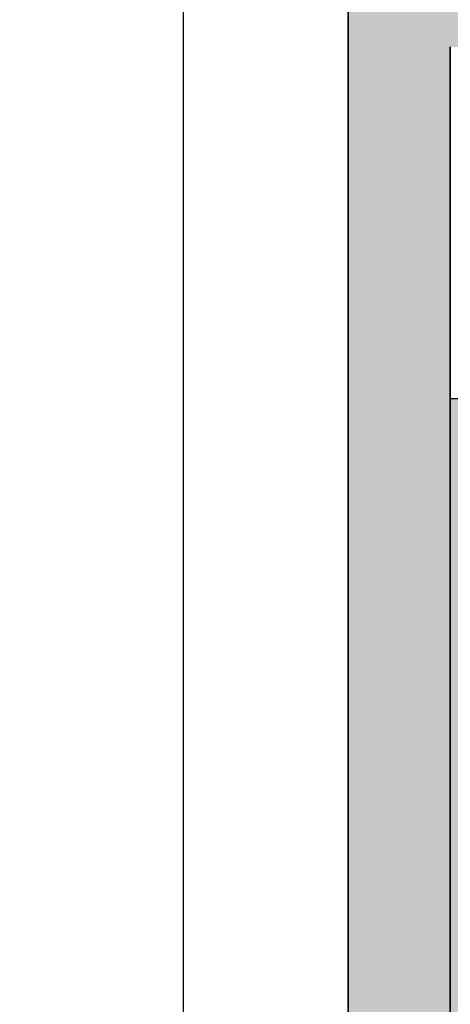
# Model space of a CAD drawing. Units: inches. Extents: x 3592 to 4861, y 1650 to 2243.
# Tile 19 of 30: x 4009 to 4047, y 2072 to 2159. Entities that reach past the tile are written whole.
import ezdxf

# ---------------------------------------------------------------- set-up
doc = ezdxf.new("R2010")
doc.units = ezdxf.units.IN
for name, color, linetype, lineweight in [('A-ANNO-DIMS', 2, 'Continuous', 13), ('A-FURN', 9, 'Continuous', 13), ('A-WALL', 7, 'Continuous', 35)]:
    doc.layers.add(name, color=color, linetype=linetype, lineweight=lineweight)
doc.layers.add('A-WALL-PATT', color=252, linetype='Continuous', lineweight=13, true_color=0x939598)
doc.layers.add('MOBIL', color=7, linetype='Continuous')
doc.styles.get("Standard").update_dxf_attribs({"font": 'arial.ttf'})
doc.dimstyles.new('ISO-25', dxfattribs={"dimtxt": 9, "dimasz": 2.5, "dimexe": 1.25, "dimexo": 0.625, "dimtad": 1, "dimlunit": 3, "dimtxsty": 'Standard', "dimcen": 2.5, "dimadec": 0, "dimazin": 0, "dimtfac": 1, "dimtmove": 0, "dimatfit": 3, "dimfxl": 1, "dimarcsym": 0})

# ---------------------------------------------------------------- blocks, each defined once
blk = doc.blocks.new('*D6')
at = {"layer": 'A-ANNO-DIMS', "color": 0, "lineweight": -2, "transparency": 16777216}
for p, q in [((4037.745, 2165.219), (4022.592, 2165.219)), ((4023.842, 2162.719), (4023.842, 1687.719)), ((4037.745, 1685.219), (4022.592, 1685.219))]:
    blk.add_line(p, q, dxfattribs=at)
at = {"layer": 'A-ANNO-DIMS', "color": 0, "transparency": 16777216}
for points in [[(4023.426, 2162.719), (4024.259, 2162.719), (4023.842, 2165.219)], [(4023.426, 1687.719), (4024.259, 1687.719), (4023.842, 1685.219)]]:
    blk.add_solid(points, dxfattribs=at)
at = {"layer": 'Defpoints', "color": 0, "transparency": 16777216}
for p in [(4038.37, 2165.219), (4023.842, 1685.219), (4038.37, 1685.219)]:
    blk.add_point(p, dxfattribs=at)
at = {"layer": 'A-ANNO-DIMS', "color": 0, "transparency": 16777216, "insert": (4018.622, 1925.219), "char_height": 9, "attachment_point": 5, "rotation": 90}
blk.add_mtext("40'", dxfattribs=at)
blk = doc.blocks.new('Aparador Aido WV')
at = {"layer": 'MOBIL'}
h = blk.add_hatch(color=256, dxfattribs=at)
h.set_gradient(color1=(226, 228, 228), one_color=1, tint=1, name='CYLINDER')
h.paths.add_polyline_path([(0.9, -0.45), (0.9, -0.43), (-0.9, -0.43), (-0.9, -0.45)])
blk.add_lwpolyline([(-0.9, -0.45), (0.9, -0.45), (0.9, 0), (-0.9, 0)], close=True, dxfattribs=at)
blk = doc.blocks.new('*D154')
at = {"layer": 'A-ANNO-DIMS', "color": 0, "lineweight": -2, "transparency": 16777216}
for p, q in [((4067.606, 2156.844), (4067.606, 2172.621)), ((4168.621, 2156.844), (4168.621, 2172.621)), ((4067.606, 2171.371), (3930.452, 2171.371)), ((4166.121, 2171.371), (4070.106, 2171.371))]:
    blk.add_line(p, q, dxfattribs=at)
at = {"layer": 'A-ANNO-DIMS', "color": 0, "transparency": 16777216}
for points in [[(4070.106, 2171.788), (4070.106, 2170.955), (4067.606, 2171.371)], [(4166.121, 2171.788), (4166.121, 2170.955), (4168.621, 2171.371)]]:
    blk.add_solid(points, dxfattribs=at)
at = {"layer": 'Defpoints', "color": 0, "transparency": 16777216}
for p in [(4067.606, 2171.371), (4067.606, 2156.219), (4168.621, 2156.219)]:
    blk.add_point(p, dxfattribs=at)
at = {"layer": 'A-ANNO-DIMS', "color": 0, "transparency": 16777216, "insert": (3997.779, 2176.653), "char_height": 9, "attachment_point": 5}
blk.add_mtext('BED GROUP 8\'-5" TYP.', dxfattribs=at)

msp = doc.modelspace()

# ---------------------------------------------------------------- hatches: boundary and pattern name
at = {"layer": 'A-WALL-PATT'}
h = msp.add_hatch(color=256, dxfattribs=at)
h.dxf.hatch_style = 1
h.paths.add_polyline_path([(4398.37, 2165.219), (4038.37, 2165.219), (4038.37, 1993.219), (4047.37, 1993.219), (4047.37, 2156.219), (4191.37, 2156.219), (4191.37, 2150.219), (4195.37, 2150.219), (4195.37, 2156.219), (4256.37, 2156.219), (4256.37, 2150.219), (4265.37, 2150.219), (4265.37, 2156.219), (4389.37, 2156.219), (4389.37, 2114.219), (4398.37, 2114.219)])
h.paths.add_polyline_path([(4265.37, 2102.219), (4256.37, 2102.219), (4256.37, 2096.219), (4195.37, 2096.219), (4195.37, 2102.219), (4191.37, 2102.219), (4191.37, 2020.219), (4195.37, 2020.219), (4195.37, 2087.219), (4256.37, 2087.219), (4256.37, 2020.219), (4306.37, 2020.219), (4306.37, 2024.219), (4265.37, 2024.219)], flags=17)
h.paths.add_polyline_path([(4398.37, 2066.219), (4389.37, 2066.219), (4389.37, 2024.219), (4348.37, 2024.219), (4348.37, 2020.219), (4389.37, 2020.219), (4389.37, 1989.719), (4398.37, 1989.719)])
h.paths.add_polyline_path([(4398.37, 1941.719), (4389.37, 1941.719), (4389.37, 1911.219), (4301.37, 1911.219), (4301.37, 1907.219), (4389.37, 1907.219), (4389.37, 1865.219), (4398.37, 1865.219)])
h.paths.add_polyline_path([(4398.37, 1817.219), (4389.37, 1817.219), (4389.37, 1775.219), (4265.37, 1775.219), (4265.37, 1911.219), (4256.37, 1911.219), (4256.37, 1817.219), (4220.87, 1817.219), (4220.87, 1808.219), (4256.37, 1808.219), (4256.37, 1766.219), (4389.37, 1766.219), (4389.37, 1694.219), (4256.37, 1694.219), (4256.37, 1685.219), (4398.37, 1685.219)])
h.paths.add_polyline_path([(4178.87, 1817.219), (4077.37, 1817.219), (4077.37, 1808.219), (4178.87, 1808.219)])
h.paths.add_polyline_path([(4111.37, 2020.219), (4155.37, 2020.219), (4155.37, 2024.219), (4077.37, 2024.219), (4077.37, 2020.219), (4107.37, 2020.219), (4107.37, 1942.219), (4047.37, 1942.219), (4047.37, 1969.219), (4038.37, 1969.219), (4038.37, 1911.219), (4047.37, 1911.219), (4047.37, 1938.219), (4107.37, 1938.219), (4107.37, 1860.219), (4077.37, 1860.219), (4077.37, 1856.219), (4111.37, 1856.219)])
h.paths.add_polyline_path([(4047.37, 1887.219), (4038.37, 1887.219), (4038.37, 1685.219), (4152.37, 1685.219), (4152.37, 1715.219), (4143.37, 1715.219), (4143.37, 1694.219), (4047.37, 1694.219)])
h.paths.add_polyline_path([(4152.37, 1772.219), (4143.37, 1772.219), (4143.37, 1751.219), (4152.37, 1751.219)], flags=17)

# ---------------------------------------------------------------- linework, layer by layer
at = {"layer": 'A-WALL'}
for p, q in [((4038.37, 1685.219), (4038.37, 2165.219)), ((4047.37, 1942.219), (4047.37, 2156.219))]:
    msp.add_line(p, q, dxfattribs=at)

# ---------------------------------------------------------------- block references
at = {"layer": 'A-FURN', "xscale": 39.3701, "yscale": 39.3701, "zscale": 39.3701, "rotation": 270}
msp.add_blockref('Aparador Aido WV', (4065.086, 2089.784), dxfattribs=at)

# ---------------------------------------------------------------- dimensions: what is measured, and where the dimension line sits
at = {"layer": 'A-ANNO-DIMS'}
dim = msp.add_linear_dim(base=(4067.606, 2171.371), p1=(4168.621, 2156.219), p2=(4067.606, 2156.219), angle=180, text='BED GROUP <> TYP.', dimstyle='ISO-25', override={"dimdec": 1, "dimlfac": 1, "dimrnd": 0, "dimzin": 1, "dimdsep": 46, "dimlunit": 4, "dimfrac": 2}, dxfattribs=at)
dim.commit()
dim.dimension.update_dxf_attribs({"geometry": '*D154', "text_midpoint": (3997.779, 2176.653)})
dim = msp.add_linear_dim(base=(4023.842, 1685.219), p1=(4038.37, 2165.219), p2=(4038.37, 1685.219), angle=90, dimstyle='ISO-25', override={"dimclrd": 0, "dimclre": 0, "dimclrt": 0}, dxfattribs=at)
dim.commit()
dim.dimension.update_dxf_attribs({"geometry": '*D6', "text_midpoint": (4018.622, 1925.219)})

doc.saveas('drawing.dxf')
